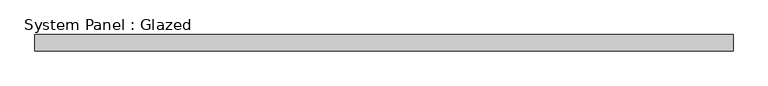
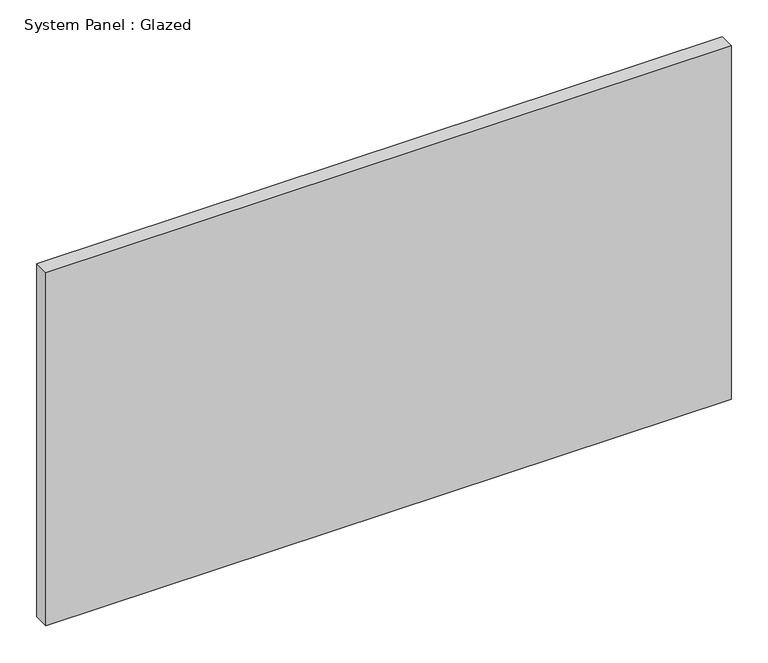
"""IFC4 building model written with IfcOpenShell, lengths in millimetres: plate geometry, System Panel : Glazed."""

from ifc_helpers import new_model, si_unit, origin, origin_with_axes, place, context, project, spatial, polyline, outline, extrude, source, transform, mapped, element, save


def system_panel_glazed_4987496d(model_context):
    return source(origin(), model_context, "Body", "SweptSolid", [
        extrude(outline(polyline([(539.75, 19.05), (-539.75, 19.05), (-539.75, 44.45), (539.75, 44.45), (539.75, 19.05)])), origin_with_axes(), (0.0, 0.0, 1.0), 588.01),
    ])


if __name__ == "__main__":
    model = new_model("IFC4")
    model_context = context("Model", 3, world=origin())
    ifc_project = project(units=[si_unit("LENGTHUNIT", "METRE", prefix="MILLI")], contexts=[model_context])
    site = spatial("IfcSite", under=ifc_project)
    building = spatial("IfcBuilding", under=site)
    placement = place(None, origin())
    system_panel_glazed_shape = system_panel_glazed_4987496d(model_context)
    element("IfcPlate", 1, ObjectType="System Panel : Glazed", at=placement, inside=building, context=model_context, shape_type="MappedRepresentation", body=[
        mapped(system_panel_glazed_shape, transform((0.0, 0.0, 0.0), x_axis=(1.0, 0.0, 0.0), y_axis=(0.0, 1.0, 0.0), z_axis=(0.0, 0.0, 1.0))),
    ])
    save(model, "model.ifc")

# Revit data of these elements
# Type "System Panel : Glazed"
#   Construction Type Id = "GSP4R"
#   Analytic Construction = "1/8 in Pilkington single glazing"
#   Visual Light Transmittance = 0.9
#   Solar Heat Gain Coefficient = 0.86
#   Heat Transfer Coefficient (U) = 1.18115 BTU/(h·ft²·°F)
#   Define Thermal Properties by = 1
# Element 1 (IfcPlate, "System Panel : Glazed")
#   Materials on its faces: "Glass"
# Materials
#   "Glass": class "Glass", colour RGB 0 128 192, transparency 0.75, Description = "Soda Lime Glass", Cost = 0
